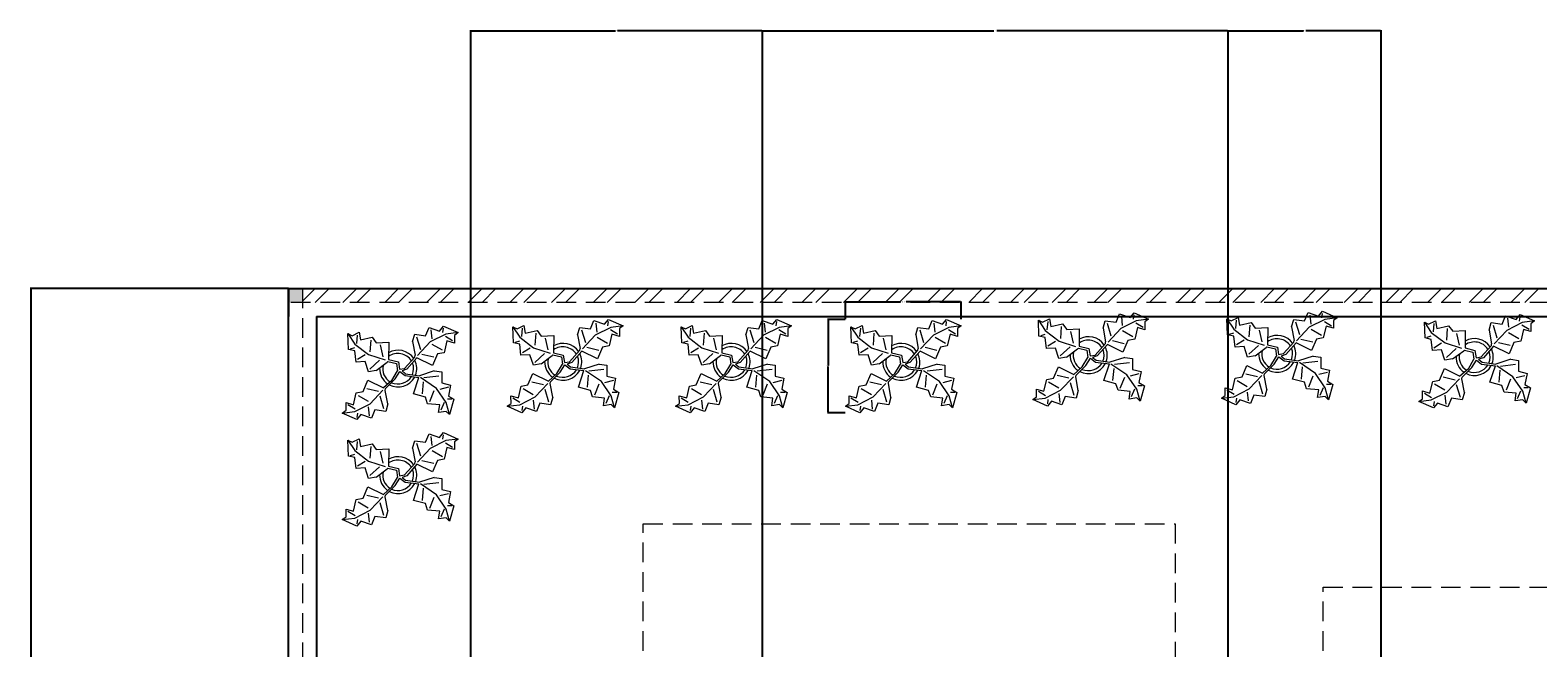
# Model space of a CAD drawing. Units: inches. Extents: x 19613 to 21413, y 12082 to 13202.
# Tile 5 of 9: x 19613 to 20100, y 13002 to 13202. Entities that reach past the tile are written whole.
import ezdxf

# ---------------------------------------------------------------- set-up
doc = ezdxf.new("R2010")
doc.units = ezdxf.units.IN
doc.linetypes.add('HIDDEN', pattern=[9.525, 6.35, -3.175])
for name, color, linetype, lineweight in [('A-ANNO-DIMS', 2, 'Continuous', 18), ('A-COLS-PATT', 6, 'Continuous', 13), ('A-FLOR-HIDN', 8, 'HIDDEN', 13), ('A-WALL-PATT', 252, 'Continuous', 13), ('C-PROP', 7, 'Continuous', 25), ('C-PROP-HIDN', 8, 'HIDDEN', 13), ('L-PLNT', 116, 'Continuous', 18)]:
    doc.layers.add(name, color=color, linetype=linetype, lineweight=lineweight)
doc.styles.get("Standard").update_dxf_attribs({"font": 'arial.ttf'})
doc.dimstyles.get("Standard").update_dxf_attribs({"dimtxt": 0.18, "dimasz": 0.18, "dimexe": 0.18, "dimexo": 0.0625, "dimgap": 0.09, "dimtad": 0, "dimtih": 1, "dimtoh": 1, "dimdec": 4, "dimzin": 0, "dimdsep": 46, "dimtxsty": 'Standard', "dimcen": 0.09, "dimadec": 0, "dimazin": 0, "dimtfac": 1, "dimtdec": 4, "dimtofl": 0, "dimtmove": 0, "dimatfit": 3, "dimfxl": 1, "dimtolj": 1, "dimtzin": 0, "dimarcsym": 0})

# ---------------------------------------------------------------- blocks, each defined once
blk = doc.blocks.new('Plant - Rubber or Philodendron')
for p, q in [((-16.2005, 11.4774), (-13.9899, 8.1064)), ((-16.2005, 11.4774), (-14.8639, 10.7964)), ((-16.0159, 6.3329), (-16.2005, 11.4774)), ((-14.8639, 10.7964), (-12.6195, 11.8975)), ((-13.3174, 8.325), (-13.0735, 11.0065)), ((-12.6195, 11.8975), (-12.1909, 9.4345)), ((-12.1909, 9.4345), (-8.3829, 10.3)), ((-8.3829, 10.3), (-7.0549, 8.501)), ((4.6914, 8.8812), (5.3859, 11.2828)), ((5.3859, 11.2828), (8.8871, 10.7908)), ((5.9878, 10.4842), (7.1971, 6.3869)), ((8.8871, 10.7908), (9.9809, 13.4933)), ((9.9809, 13.4933), (13.3837, 12.301)), ((15.3859, 11.3055), (10.3916, 8.7942)), ((10.5828, 12.6946), (10.8893, 9.7953)), ((13.3837, 12.301), (14.68, 13.9039)), ((14.5816, 13.2037), (14.3848, 11.8033)), ((14.68, 13.9039), (19.3848, 11.8146)), ((15.2875, 10.6053), (17.5907, 9.2105)), ((19.3848, 11.8146), (15.3859, 11.3055)), ((19.3848, 11.8146), (18.1868, 10.9119)), ((18.1868, 10.9119), (18.1925, 8.4119)), ((-14.0069, 5.8704), (-16.0159, 6.3329)), ((-15.3434, 6.5514), (-13.9984, 6.9884)), ((-13.5868, 2.2894), (-14.0069, 5.8704)), ((-13.9899, 8.1064), (-9.5434, 4.7185)), ((-8.8369, 9.409), (-9.0894, 5.6095)), ((-7.0549, 8.501), (-3.0284, 8.6941)), ((-4.8529, 4.012), (-5.7184, 7.82)), ((-3.0284, 8.6941), (-3.0709, 3.1041)), ((4.6914, 8.8812), (5.5014, 4.4831)), ((10.3916, 8.7942), (6.2847, 4.4028)), ((7.7005, 4.8881), (11.5025, 3.9967)), ((14.2977, 6.1031), (10.9934, 7.9956)), ((12.7005, 4.8994), (11.1089, 1.1958)), ((14.8995, 5.3044), (12.7005, 4.8994)), ((15.7909, 9.1065), (14.8995, 5.3044)), ((18.1925, 8.4119), (15.7909, 9.1065)), ((-10.6784, 2.491), (-13.5868, 2.2894)), ((-13.1329, 3.1804), (-10.6614, 4.727)), ((-9.5858, -0.8715), (-10.6784, 2.491)), ((-9.5434, 4.7185), (-4.1917, 2.9888)), ((-9.1318, 0.0195), (-5.9793, 2.9025)), ((-7.1228, -0.443), (-3.5248, 2.2131)), ((-3.5248, 2.2131), (-3.3011, 2.4355)), ((-3.3011, 2.4355), (-0.5306, 1.7947)), ((-3.0709, 3.1041), (0.0797, 2.3163)), ((-0.5306, 1.7947), (-0.2255, -0.5527)), ((-0.5306, 1.7947), (-0.5306, 1.7947)), ((0.0797, 2.3163), (0.4866, -0.031)), ((0.4866, -0.031), (2.1141, 0.2298)), ((2.1141, 0.2298), (5.4346, 3.9146)), ((6.1032, 3.6844), (2.8262, -0.031)), ((5.4346, 3.9146), (5.5014, 4.4831)), ((11.1089, 1.1958), (6.1032, 3.6844)), ((-11.3237, -7.2629), (-9.7321, -3.5593)), ((-9.7321, -3.5593), (-4.7264, -6.0479)), ((-7.1228, -0.443), (-9.5858, -0.8715)), ((-2.019, -3.6148), (-4.7264, -6.0479)), ((-4.0579, -6.2781), (-0.9375, -3.1608)), ((-2.019, -3.6148), (-0.2255, -0.5527)), ((-0.9375, -3.1608), (0.5883, -0.8135)), ((0.5883, -0.8135), (2.2447, -2.0916)), ((2.8262, -0.031), (1.3003, -0.5527)), ((1.3003, -0.5527), (2.4193, -1.4655)), ((2.2447, -2.0916), (6.7108, -2.6626)), ((2.4193, -1.4655), (6.895, -2.1175)), ((4.943, -7.9659), (6.7108, -2.6626)), ((11.6605, -0.5413), (6.895, -2.1175)), ((12.3677, -6.1981), (7.219, -2.6772)), ((8.125, -4.0768), (7.7715, -7.9659)), ((8.3544, -2.7453), (13.1973, -2.1704)), ((11.6605, -0.5413), (14.1354, -0.8948)), ((14.1354, -0.8948), (14.1354, -4.4304)), ((14.1354, -4.4304), (16.9638, -5.1375)), ((-14.4141, -11.4699), (-13.5228, -7.6679)), ((-13.5228, -7.6679), (-11.3237, -7.2629)), ((-12.921, -8.4665), (-9.6166, -10.359)), ((-6.3237, -7.2516), (-10.1257, -6.3602)), ((-9.0148, -11.1577), (-4.9047, -6.8122)), ((-4.611, -12.8477), (-5.8203, -8.7504)), ((-4.1246, -6.8466), (-4.0579, -6.2781)), ((-3.3146, -11.2447), (-4.1246, -6.8466)), ((8.8321, -9.0266), (4.943, -7.9659)), ((9.5392, -11.1479), (8.8321, -9.0266)), ((10.2463, -10.4408), (11.6605, -6.9053)), ((15.5496, -10.7943), (12.3677, -6.1981)), ((16.2567, -5.8446), (13.4283, -6.5517)), ((17.3174, -9.7337), (15.9032, -9.7337)), ((16.9638, -5.1375), (16.2567, -8.673)), ((16.2567, -8.673), (18.0245, -9.7337)), ((18.0245, -9.7337), (16.6103, -14.6834)), ((-18.008, -14.1781), (-16.8101, -13.2754)), ((-18.008, -14.1781), (-14.0091, -13.669)), ((-13.3032, -16.2674), (-18.008, -14.1781)), ((-16.8157, -10.7754), (-14.4141, -11.4699)), ((-16.8101, -13.2754), (-16.8157, -10.7754)), ((-13.9107, -12.9688), (-16.2139, -11.574)), ((-14.0091, -13.669), (-9.0148, -11.1577)), ((-13.2048, -15.5672), (-13.008, -14.1668)), ((-9.206, -15.0581), (-9.5126, -12.1588)), ((-7.5103, -13.1543), (-8.6042, -15.8568)), ((-4.0092, -13.6463), (-7.5103, -13.1543)), ((-3.3146, -11.2447), (-4.0092, -13.6463)), ((13.4283, -11.5015), (9.5392, -11.1479)), ((13.0748, -13.9763), (13.4283, -11.5015)), ((15.5496, -13.6228), (13.0748, -13.9763)), ((14.8425, -10.7943), (13.7819, -13.2692)), ((16.6103, -14.6834), (15.5496, -10.7943)), ((16.6103, -14.6834), (15.5496, -13.6228)), ((-12.0069, -14.6645), (-13.3032, -16.2674)), ((-8.6042, -15.8568), (-12.0069, -14.6645))]:
    blk.add_line(p, q)
for centre, radius, start, end in [((0, 0), 6.1275, 34.37569, 120.1028), ((-0.0601, -0.2075), 5.2461, 33.82192, 124.9414), ((0.0308, 0.1664), 6, 178.6147, 235.1169), ((0.0308, 0.1664), 5, 168.1647, 238.6725), ((-0.2664, 0.1682), 5.2775, 338.4094, 20.03007), ((-0.098, 0.1364), 6.1288, 341.2017, 26.09184), ((-0.0234, 0.3825), 6.1492, 242.5812, 331.2714), ((-0.1102, 0.4886), 5.2883, 247.3711, 327.472)]:
    blk.add_arc(centre, radius, start, end)
blk = doc.blocks.new('*D39')
at = {"layer": 'A-ANNO-DIMS', "color": 0, "lineweight": -2, "transparency": 16777216}
for p, q in [((19876.51, 13108.39), (19876.51, 13114.12)), ((19876.69, 13113.94), (19894.24, 13113.94)), ((19913.72, 13113.94), (19896.17, 13113.94)), ((19913.9, 13108.39), (19913.9, 13114.12))]:
    blk.add_line(p, q, dxfattribs=at)
at = {"layer": 'A-ANNO-DIMS', "color": 0, "transparency": 16777216}
for points in [[(19876.69, 13113.97), (19876.69, 13113.91), (19876.51, 13113.94)], [(19913.72, 13113.97), (19913.72, 13113.91), (19913.9, 13113.94)]]:
    blk.add_solid(points, dxfattribs=at)
at = {"layer": 'Defpoints', "color": 0, "transparency": 16777216}
for p in [(19913.9, 13113.94), (19876.51, 13108.33), (19913.9, 13108.33)]:
    blk.add_point(p, dxfattribs=at)
at = {"layer": 'A-ANNO-DIMS', "color": 0, "transparency": 16777216, "insert": (19895.2, 13113.94), "char_height": 0.18, "attachment_point": 5}
blk.add_mtext('\\A1;PLANT 37 TYP.', dxfattribs=at)
blk = doc.blocks.new('*D40')
at = {"layer": 'A-ANNO-DIMS', "color": 0, "lineweight": -2, "transparency": 16777216}
for p, q in [((19876.44, 13108.33), (19870.72, 13108.33)), ((19870.9, 13108.15), (19870.9, 13093.43)), ((19870.9, 13078.34), (19870.9, 13093.06)), ((19876.44, 13078.16), (19870.72, 13078.16))]:
    blk.add_line(p, q, dxfattribs=at)
at = {"layer": 'A-ANNO-DIMS', "color": 0, "transparency": 16777216}
for points in [[(19870.87, 13108.15), (19870.93, 13108.15), (19870.9, 13108.33)], [(19870.87, 13078.34), (19870.93, 13078.34), (19870.9, 13078.16)]]:
    blk.add_solid(points, dxfattribs=at)
at = {"layer": 'Defpoints', "color": 0, "transparency": 16777216}
for p in [(19870.9, 13108.33), (19876.51, 13108.33), (19876.51, 13078.16)]:
    blk.add_point(p, dxfattribs=at)
at = {"layer": 'A-ANNO-DIMS', "color": 0, "transparency": 16777216, "insert": (19870.9, 13093.25), "char_height": 0.18, "attachment_point": 5}
blk.add_mtext('\\A1;30 TYP.', dxfattribs=at)
blk = doc.blocks.new('*D84')
at = {"layer": 'A-ANNO-DIMS', "color": 0, "lineweight": -2, "transparency": 16777216}
for p, q in [((19696.63, 13118.28), (19613.26, 13118.28)), ((19613.44, 13118.1), (19613.44, 12646.96)), ((19613.44, 12175.46), (19613.44, 12646.6)), ((19696.63, 12175.28), (19613.26, 12175.28))]:
    blk.add_line(p, q, dxfattribs=at)
at = {"layer": 'A-ANNO-DIMS', "color": 0, "transparency": 16777216}
for points in [[(19613.41, 13118.1), (19613.47, 13118.1), (19613.44, 13118.28)], [(19613.41, 12175.46), (19613.47, 12175.46), (19613.44, 12175.28)]]:
    blk.add_solid(points, dxfattribs=at)
at = {"layer": 'Defpoints', "color": 0, "transparency": 16777216}
for p in [(19613.44, 13118.28), (19696.69, 13118.28), (19696.69, 12175.28)]:
    blk.add_point(p, dxfattribs=at)
at = {"layer": 'A-ANNO-DIMS', "color": 0, "transparency": 16777216, "insert": (19613.44, 12646.78), "char_height": 0.18, "attachment_point": 5}
blk.add_mtext('\\A1;943', dxfattribs=at)
blk = doc.blocks.new('*D101')
at = {"layer": 'A-ANNO-DIMS', "color": 0, "lineweight": -2, "transparency": 16777216}
for p, q in [((19755.54, 12982.34), (19755.54, 13201.71)), ((19755.72, 13201.53), (19802.31, 13201.53)), ((19849.55, 13201.53), (19802.96, 13201.53)), ((19849.73, 12982.34), (19849.73, 13201.71))]:
    blk.add_line(p, q, dxfattribs=at)
at = {"layer": 'A-ANNO-DIMS', "color": 0, "transparency": 16777216}
for points in [[(19755.72, 13201.56), (19755.72, 13201.5), (19755.54, 13201.53)], [(19849.55, 13201.56), (19849.55, 13201.5), (19849.73, 13201.53)]]:
    blk.add_solid(points, dxfattribs=at)
at = {"layer": 'Defpoints', "color": 0, "transparency": 16777216}
for p in [(19849.73, 13201.53), (19755.54, 12982.28), (19849.73, 12982.28)]:
    blk.add_point(p, dxfattribs=at)
at = {"layer": 'A-ANNO-DIMS', "color": 0, "transparency": 16777216, "insert": (19802.63, 13201.53), "char_height": 0.18, "attachment_point": 5}
blk.add_mtext('\\A1;94.2', dxfattribs=at)
blk = doc.blocks.new('*D102')
at = {"layer": 'A-ANNO-DIMS', "color": 0, "lineweight": -2, "transparency": 16777216}
for p, q in [((19849.73, 12982.34), (19849.73, 13201.71)), ((19849.91, 13201.53), (19924.46, 13201.53)), ((19999.93, 13201.53), (19925.37, 13201.53)), ((20000.11, 12982.34), (20000.11, 13201.71))]:
    blk.add_line(p, q, dxfattribs=at)
at = {"layer": 'A-ANNO-DIMS', "color": 0, "transparency": 16777216}
for points in [[(19849.91, 13201.56), (19849.91, 13201.5), (19849.73, 13201.53)], [(19999.93, 13201.56), (19999.93, 13201.5), (20000.11, 13201.53)]]:
    blk.add_solid(points, dxfattribs=at)
at = {"layer": 'Defpoints', "color": 0, "transparency": 16777216}
for p in [(20000.11, 13201.53), (19849.73, 12982.28), (20000.11, 12982.28)]:
    blk.add_point(p, dxfattribs=at)
at = {"layer": 'A-ANNO-DIMS', "color": 0, "transparency": 16777216, "insert": (19924.92, 13201.53), "char_height": 0.18, "attachment_point": 5}
blk.add_mtext('\\A1;150.37', dxfattribs=at)
blk = doc.blocks.new('*D103')
at = {"layer": 'A-ANNO-DIMS', "color": 0, "lineweight": -2, "transparency": 16777216}
for p, q in [((20000.11, 12982.34), (20000.11, 13201.71)), ((20000.29, 13201.53), (20024.4, 13201.53)), ((20049.3, 13201.53), (20025.19, 13201.53)), ((20049.48, 12982.34), (20049.48, 13201.71))]:
    blk.add_line(p, q, dxfattribs=at)
at = {"layer": 'A-ANNO-DIMS', "color": 0, "transparency": 16777216}
for points in [[(20000.29, 13201.56), (20000.29, 13201.5), (20000.11, 13201.53)], [(20049.3, 13201.56), (20049.3, 13201.5), (20049.48, 13201.53)]]:
    blk.add_solid(points, dxfattribs=at)
at = {"layer": 'Defpoints', "color": 0, "transparency": 16777216}
for p in [(20049.48, 13201.53), (20000.11, 12982.28), (20049.48, 12982.28)]:
    blk.add_point(p, dxfattribs=at)
at = {"layer": 'A-ANNO-DIMS', "color": 0, "transparency": 16777216, "insert": (20024.79, 13201.53), "char_height": 0.18, "attachment_point": 5}
blk.add_mtext('\\A1;49.37', dxfattribs=at)

msp = doc.modelspace()

# ---------------------------------------------------------------- hatches: boundary and pattern name
at = {"layer": 'A-COLS-PATT'}
h = msp.add_hatch(color=256, dxfattribs=at)
h.dxf.hatch_style = 1
h.paths.add_polyline_path([(19701.1937, 13118.279), (19696.6937, 13118.279), (19696.6937, 13113.779), (19701.1937, 13113.779)])
h.paths.add_polyline_path([(19714.6694, 12982.279), (19705.6937, 12982.279), (19705.6937, 12973.279), (19714.6694, 12973.279)])
h.paths.add_polyline_path([(19827.1183, 12982.279), (19818.1183, 12982.279), (19818.1183, 12973.279), (19827.1183, 12973.279)])
h.paths.add_polyline_path([(19982.6937, 12982.279), (19973.6937, 12982.279), (19973.6937, 12973.279), (19982.6937, 12973.279)])
h.paths.add_polyline_path([(19982.6937, 12817.279), (19973.6937, 12817.279), (19973.6937, 12808.279), (19982.6937, 12808.279)])
h.paths.add_polyline_path([(19795.361, 12817.279), (19786.361, 12817.279), (19786.361, 12808.279), (19795.361, 12808.279)])
h.paths.add_polyline_path([(19705.6937, 12817.279), (19702.0819, 12817.279), (19702.0819, 12808.279), (19705.6937, 12808.279)])
h.paths.add_polyline_path([(19711.0819, 12817.279), (19705.6937, 12817.279), (19705.6937, 12808.279), (19711.0819, 12808.279)])
h.paths.add_polyline_path([(19714.6136, 12634.279), (19705.6937, 12634.279), (19705.6937, 12625.279), (19714.6136, 12625.279)])
h.paths.add_polyline_path([(19705.6937, 12485.8897), (19701.1937, 12485.8897), (19701.1937, 12476.8897), (19705.6937, 12476.8897)])
h.paths.add_polyline_path([(19709.3479, 12485.8897), (19705.6937, 12485.8897), (19705.6937, 12476.8897), (19709.3479, 12476.8897)])
h.paths.add_polyline_path([(19701.1937, 12485.8897), (19700.3479, 12485.8897), (19700.3479, 12476.8897), (19701.1937, 12476.8897)])
h.paths.add_polyline_path([(20218.6937, 12421.279), (20209.6937, 12421.279), (20209.6937, 12412.279), (20218.6937, 12412.279)])
h.paths.add_polyline_path([(20218.6937, 12634.279), (20209.6937, 12634.279), (20209.6937, 12625.279), (20218.6937, 12625.279)])
h.paths.add_polyline_path([(20218.6937, 12808.279), (20209.6937, 12808.279), (20209.6937, 12803.279), (20218.6937, 12803.279)])
h.paths.add_polyline_path([(20218.6937, 12810.1878), (20209.6937, 12810.1878), (20209.6937, 12808.279), (20218.6937, 12808.279)])
h.paths.add_polyline_path([(20218.6937, 12803.279), (20209.6937, 12803.279), (20209.6937, 12801.1878), (20218.6937, 12801.1878)])
h.paths.add_polyline_path([(20218.6937, 12982.279), (20209.6937, 12982.279), (20209.6937, 12973.279), (20218.6937, 12973.279)])
h.paths.add_polyline_path([(20100.1214, 12982.279), (20080.8386, 12982.279), (20080.8386, 12973.279), (20091.6937, 12973.279), (20100.1214, 12973.279), (20100.1214, 12976.279)])
h.paths.add_polyline_path([(19851.5503, 12631.279), (19851.5503, 12634.279), (19828.8814, 12634.279), (19828.8814, 12625.279), (19851.5503, 12625.279)])
at = {"layer": 'A-WALL-PATT'}
h = msp.add_hatch(dxfattribs=at)
h.set_pattern_fill('ANSI32', color=256)
h.paths.add_polyline_path([(20223.1937, 13118.279), (20218.6937, 13118.279), (19701.1937, 13118.279), (19701.1937, 13113.779), (20223.1937, 13113.779)])
h.paths.add_polyline_path([(19849.7315, 12982.279), (19799.9854, 12982.279), (19799.9854, 12973.279), (19849.7315, 12973.279)])
h.paths.add_polyline_path([(19755.5378, 12982.279), (19705.6937, 12982.279), (19705.6937, 12973.279), (19755.5378, 12973.279)])
h.paths.add_polyline_path([(20000.1054, 12982.279), (19950.0534, 12982.279), (19950.0534, 12974.1171), (19950.0534, 12973.279), (20000.1054, 12973.279)])
h.paths.add_polyline_path([(20049.4797, 12982.279), (20030.7476, 12982.279), (20030.7476, 12973.279), (20049.4797, 12973.279)])
h.paths.add_polyline_path([(20100.1214, 12982.279), (20080.8386, 12982.279), (20080.8386, 12973.279), (20100.1214, 12973.279), (20100.1214, 12976.279)])
h.paths.add_polyline_path([(20218.6937, 12982.279), (20167.6937, 12982.279), (20140.1214, 12982.279), (20140.1214, 12976.279, -0.01769781), (20140.0212, 12973.45), (20167.6937, 12973.279), (20176.6937, 12973.279), (20218.6937, 12973.279)])
h.paths.add_polyline_path([(19851.5503, 12814.279), (19851.5503, 12817.279), (19793.6937, 12817.279), (19789.6937, 12817.279), (19705.6937, 12817.279), (19705.6937, 12808.279), (19851.5503, 12808.279)])
h.paths.add_polyline_path([(19982.6937, 12973.279), (19973.6937, 12973.279), (19973.6937, 12817.279), (19887.5503, 12817.279), (19887.5503, 12808.279), (19973.6937, 12808.279), (19982.6937, 12808.279)])
h.paths.add_polyline_path([(20058.6937, 12850.5529), (19982.6937, 12850.5529), (19982.6937, 12846.5529), (20058.6937, 12846.5529)])
h.paths.add_polyline_path([(20095.6937, 12973.279), (20091.6937, 12973.279), (20091.6937, 12850.5529), (20087.6937, 12850.5529), (20087.6937, 12846.5529), (20095.6937, 12846.5529)])
h.paths.add_polyline_path([(20218.6937, 12808.279), (20140.8605, 12808.279), (20126.9413, 12808.279), (20126.9413, 12803.279), (20140.8605, 12803.279), (20218.6937, 12803.279)])
h.paths.add_polyline_path([(19738.3931, 12634.279), (19705.6937, 12634.279), (19705.6937, 12625.279), (19738.3931, 12625.279)])
h.paths.add_polyline_path([(19912.6937, 12634.279), (19903.6937, 12634.279), (19891.5503, 12634.279), (19891.5503, 12625.279), (19903.6937, 12625.279), (19903.6937, 12445.279), (19975.6937, 12445.279), (20128.6937, 12445.279), (20128.6937, 12412.279), (20149.8479, 12412.279), (20149.8479, 12421.279), (20137.6937, 12421.279), (20137.6937, 12454.279), (20137.6937, 12580.2801), (20133.6937, 12580.2801), (20133.6937, 12454.279), (19984.6937, 12454.279), (19984.6937, 12625.279), (19993.6937, 12625.279), (19993.6937, 12634.279), (19984.6937, 12634.279), (19975.6937, 12634.279), (19975.6937, 12454.279), (19912.6937, 12454.279)])
h.paths.add_polyline_path([(20218.6937, 12634.279), (20137.6937, 12634.279), (20029.6937, 12634.279), (20029.6937, 12625.279), (20137.6937, 12625.279), (20218.6937, 12625.279)])
h.paths.add_polyline_path([(21014.4339, 12634.279), (21005.4339, 12634.279), (20993.2905, 12634.279), (20993.2905, 12625.279), (21005.4339, 12625.279), (21005.4339, 12445.279), (21077.4339, 12445.279), (21230.4339, 12445.279), (21230.4339, 12412.279), (21251.5881, 12412.279), (21251.5881, 12421.279), (21239.4339, 12421.279), (21239.4339, 12454.279), (21239.4339, 12580.2801), (21235.4339, 12580.2801), (21235.4339, 12454.279), (21086.4339, 12454.279), (21086.4339, 12625.279), (21095.4339, 12625.279), (21095.4339, 12634.279), (21086.4339, 12634.279), (21077.4339, 12634.279), (21077.4339, 12454.279), (21014.4339, 12454.279)])
h.paths.add_polyline_path([(20840.1333, 12634.279), (20807.4339, 12634.279), (20807.4339, 12625.279), (20840.1333, 12625.279)])
h.paths.add_polyline_path([(20953.2905, 12631.279), (20953.2905, 12634.279), (20930.6216, 12634.279), (20930.6216, 12625.279), (20953.2905, 12625.279)])
h.paths.add_polyline_path([(21320.4339, 12634.279), (21239.4339, 12634.279), (21131.4339, 12634.279), (21131.4339, 12625.279), (21239.4339, 12625.279), (21320.4339, 12625.279)])
h.paths.add_polyline_path([(21084.4339, 12973.279), (21075.4339, 12973.279), (21075.4339, 12817.279), (20989.2905, 12817.279), (20989.2905, 12808.279), (21075.4339, 12808.279), (21084.4339, 12808.279)])
h.paths.add_polyline_path([(21142.1261, 12863.2893), (21084.4339, 12863.2893), (21084.4339, 12846.5529), (21142.1261, 12846.5529)])
h.paths.add_polyline_path([(21320.4339, 12808.279), (21242.6007, 12808.279), (21228.6815, 12808.279), (21228.6815, 12803.279), (21242.6007, 12803.279), (21320.4339, 12803.279)])
h.paths.add_polyline_path([(20857.278, 12982.279), (20807.4339, 12982.279), (20807.4339, 12973.279), (20857.278, 12973.279)])
h.paths.add_polyline_path([(20951.4717, 12982.279), (20901.7255, 12982.279), (20901.7255, 12973.279), (20951.4717, 12973.279)])
h.paths.add_polyline_path([(21101.8455, 12982.279), (21051.7936, 12982.279), (21051.7936, 12974.1171), (21051.7936, 12973.279), (21101.8455, 12973.279)])
h.paths.add_polyline_path([(21151.2199, 12982.279), (21132.4878, 12982.279), (21132.4878, 12973.279), (21151.2199, 12973.279)])
h.paths.add_polyline_path([(21201.8616, 12982.279), (21182.5788, 12982.279), (21182.5788, 12973.279), (21193.4339, 12973.279), (21201.8616, 12973.279), (21201.8616, 12976.279)])
h.paths.add_polyline_path([(21320.4339, 12982.279), (21269.4339, 12982.279), (21241.8616, 12982.279), (21241.8616, 12976.279, -0.01769781), (21241.7614, 12973.45), (21269.4339, 12973.279), (21278.4339, 12973.279), (21320.4339, 12973.279)])
h.paths.add_polyline_path([(20953.2905, 12817.279), (20895.4339, 12817.279), (20891.4339, 12817.279), (20807.4339, 12817.279), (20807.4339, 12808.279), (20953.2905, 12808.279)])
h.paths.add_polyline_path([(21197.4339, 12973.279), (21193.4339, 12973.279), (21193.4339, 12850.5529), (21197.4339, 12850.5529)])
h.paths.add_polyline_path([(21320.4339, 12550.279), (21272.5278, 12550.279), (21272.5278, 12546.279), (21320.4339, 12546.279)])
h.paths.add_polyline_path([(21320.4339, 12421.279), (21283.2222, 12421.279), (21283.2222, 12412.279), (21320.4339, 12412.279)])

# ---------------------------------------------------------------- linework, layer by layer
at = {"layer": 'A-FLOR-HIDN'}
for p, q in [((19811.233, 12982.279), (19811.233, 13042.279)), ((19811.233, 13042.279), (19982.958, 13042.279)), ((19982.958, 13042.279), (19982.958, 12982.279)), ((20030.7476, 12982.279), (20030.7476, 13021.8552)), ((20030.7476, 13021.8552), (20218.6937, 13021.8552))]:
    msp.add_line(p, q, dxfattribs=at)
at = {"layer": 'C-PROP'}
for p, q in [((19696.6937, 13118.279), (20227.6937, 13118.279)), ((19696.6937, 12175.279), (19696.6937, 13118.279)), ((19696.6937, 13118.279), (19696.6937, 13109.279)), ((19696.6937, 13118.279), (19705.6937, 13118.279)), ((19696.6937, 13118.279), (19701.1937, 13118.279)), ((19705.6937, 13109.279), (20218.6937, 13109.279)), ((19705.6937, 13109.279), (19705.6937, 12184.279))]:
    msp.add_line(p, q, dxfattribs=at)
at = {"layer": 'C-PROP-HIDN'}
for p, q in [((19701.1937, 13118.279), (19701.1937, 12175.279)), ((20227.6937, 13113.779), (19696.6937, 13113.779))]:
    msp.add_line(p, q, dxfattribs=at)

# ---------------------------------------------------------------- block references
at = {"layer": 'L-PLNT'}
for p in [(19785.3321, 13094.4272), (19839.6922, 13094.4272), (19894.5151, 13094.4272), (19955.036, 13096.5799), (20015.9194, 13097.0313), (20079.702, 13095.9866), (19732.0591, 13092.2549), (19732.0591, 13057.8591)]:
    msp.add_blockref('Plant - Rubber or Philodendron', p, dxfattribs=at)

# ---------------------------------------------------------------- dimensions: what is measured, and where the dimension line sits
at = {"layer": 'A-ANNO-DIMS'}
for base, p1, p2, override, picture, middle in [((19849.7315, 13201.529), (19755.5378, 12982.279), (19849.7315, 12982.279), {"dimdec": 1, "dimlfac": 1, "dimrnd": 0, "dimzin": 0, "dimdsep": 46, "dimlunit": 2}, '*D101', (19802.6347, 13201.529)), ((20000.1054, 13201.529), (19849.7315, 12982.279), (20000.1054, 12982.279), {"dimdec": 2, "dimlfac": 1, "dimrnd": 0, "dimzin": 0, "dimdsep": 46, "dimlunit": 2}, '*D102', (19924.9185, 13201.529)), ((20049.4797, 13201.529), (20000.1054, 12982.279), (20049.4797, 12982.279), {"dimdec": 2, "dimlfac": 1, "dimrnd": 0, "dimzin": 0, "dimdsep": 46, "dimlunit": 2}, '*D103', (20024.7925, 13201.529))]:
    dim = msp.add_linear_dim(base=base, p1=p1, p2=p2, dimstyle='Standard', override=override, dxfattribs=at)
    dim.commit()
    dim.dimension.update_dxf_attribs({"geometry": picture, "text_midpoint": middle})
dim = msp.add_linear_dim(base=(19613.4437, 13118.279), p1=(19696.6937, 12175.279), p2=(19696.6937, 13118.279), angle=90, dimstyle='Standard', override={"dimdec": 0, "dimlfac": 1, "dimrnd": 0, "dimzin": 0, "dimdsep": 46, "dimlunit": 2}, dxfattribs=at)
dim.commit()
dim.dimension.update_dxf_attribs({"geometry": '*D84', "text_midpoint": (19613.4437, 12646.779)})
dim = msp.add_linear_dim(base=(19913.8999, 13113.94), p1=(19876.5071, 13108.3311), p2=(19913.8999, 13108.3311), text='PLANT <> TYP.', dimstyle='Standard', override={"dimdec": 0, "dimlfac": 1, "dimrnd": 0, "dimzin": 0, "dimdsep": 46, "dimlunit": 2}, dxfattribs=at)
dim.commit()
dim.dimension.update_dxf_attribs({"geometry": '*D39', "text_midpoint": (19895.2035, 13113.94)})
dim = msp.add_linear_dim(base=(19870.8981, 13108.3311), p1=(19876.5071, 13078.1598), p2=(19876.5071, 13108.3311), angle=90, text='<> TYP.', dimstyle='Standard', override={"dimdec": 0, "dimlfac": 1, "dimrnd": 0, "dimzin": 0, "dimdsep": 46, "dimlunit": 2}, dxfattribs=at)
dim.commit()
dim.dimension.update_dxf_attribs({"geometry": '*D40', "text_midpoint": (19870.8981, 13093.2455)})

doc.saveas('drawing.dxf')
